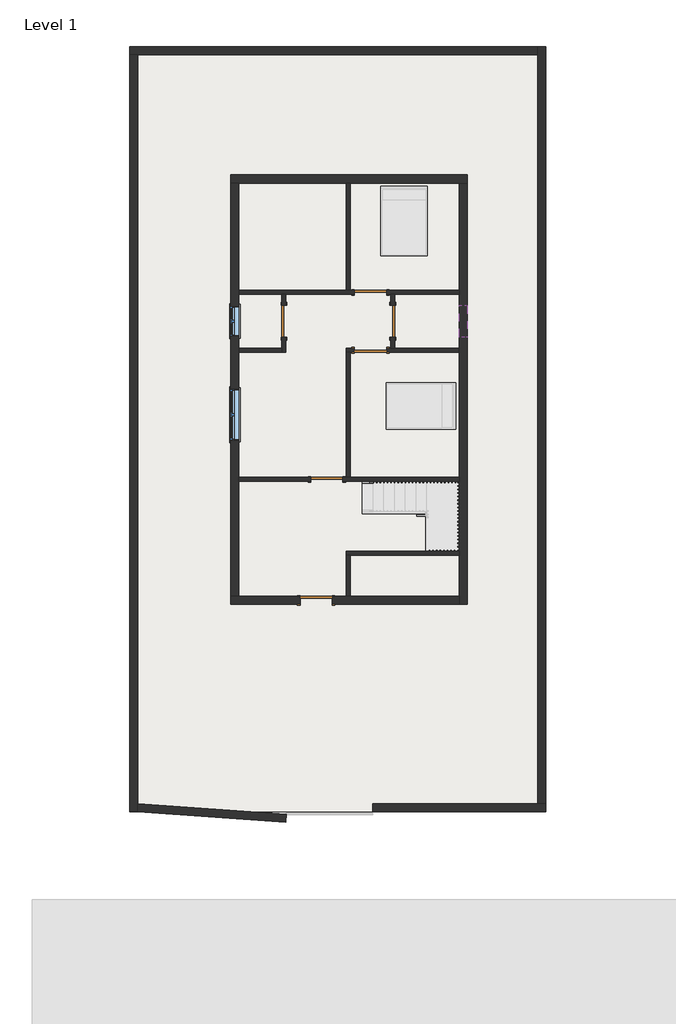
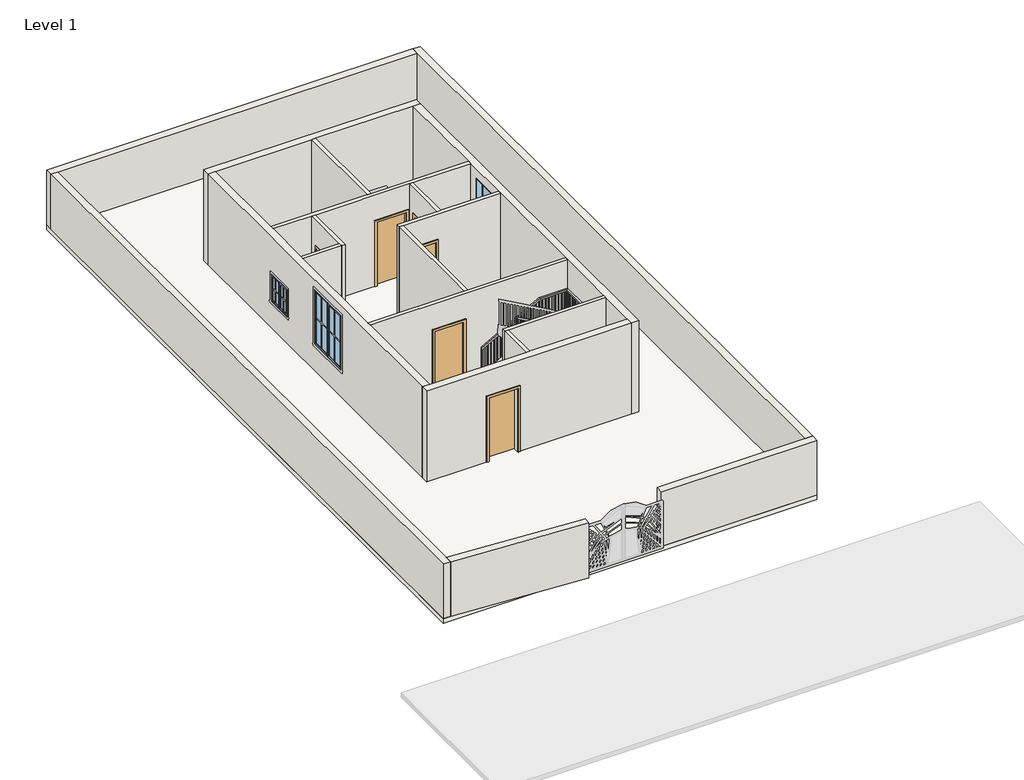
# One storey, part 1 of 2: 19 walls, 6 doors, 3 windows, 1 railing, 1 slab.
"""IFC4 building model written with IfcOpenShell, lengths in millimetres."""

from ifc_helpers import new_model, si_unit, frame, origin, origin_with_axes, place, context, project, spatial, polyline, outline, extrude, faceted_brep, transform, mapped, element, save
from components import door_305aa2a5, door_e5f9f3c4, door_a90ba1ad, window_c1f32544, window_339605e1, window_9ac97e1a

model = new_model("IFC4")

# Units and contexts
model_context = context("Model", 3, world=origin())
ifc_project = project(units=[si_unit("LENGTHUNIT", "METRE", prefix="MILLI")], contexts=[model_context])

# Site, building, storey
site = spatial("IfcSite", under=ifc_project)
building = spatial("IfcBuilding", under=site)
storey = spatial("IfcBuildingStorey", under=building, Name="Level 1", Elevation=0.0)

# Doors
placement = place(None, origin())
door_shape = door_305aa2a5(model_context)
element("IfcDoor", 1, ObjectType="Single-Flush : 36\" x 84\"", at=placement, inside=storey, context=model_context, shape_type="MappedRepresentation", body=[
    mapped(door_shape, transform((-650.940747, 3300.4435985, 0.0), x_axis=(-1.0, 0.0, 0.0), y_axis=(0.0, -1.0, 0.0), z_axis=(0.0, 0.0, 1.0))),
])
element("IfcDoor", 2, ObjectType="Single-Flush : 36\" x 84\"", at=placement, inside=storey, context=model_context, shape_type="MappedRepresentation", body=[
    mapped(door_shape, transform((-22.290747, 2481.2935985, 0.0), x_axis=(0.0, 1.0, 0.0), y_axis=(-1.0, 0.0, 0.0), z_axis=(0.0, 0.0, 1.0))),
])
door_2_shape = door_e5f9f3c4(model_context)
element("IfcDoor", 3, ObjectType="Single-Flush : 36\" x 84\"", at=placement, inside=storey, context=model_context, shape_type="MappedRepresentation", body=[
    mapped(door_2_shape, transform((-650.940747, 1662.1435985, 0.0), x_axis=(-1.0, 0.0, 0.0), y_axis=(0.0, -1.0, 0.0), z_axis=(0.0, 0.0, 1.0))),
])
element("IfcDoor", 4, ObjectType="Single-Flush : 36\" x 84\"", at=placement, inside=storey, context=model_context, shape_type="MappedRepresentation", body=[
    mapped(door_2_shape, transform((-3108.390747, 2481.2935985, 0.0), x_axis=(0.0, 1.0, 0.0), y_axis=(-1.0, 0.0, 0.0), z_axis=(0.0, 0.0, 1.0))),
])
element("IfcDoor", 5, ObjectType="Single-Flush : 36\" x 84\"", at=placement, inside=storey, context=model_context, shape_type="MappedRepresentation", body=[
    mapped(door_2_shape, transform((-1889.190747, -2008.1564015, 0.0), x_axis=(1.0, 0.0, 0.0), y_axis=(0.0, 1.0, 0.0), z_axis=(0.0, 0.0, 1.0))),
])
door_3_shape = door_a90ba1ad(model_context)
element("IfcDoor", 6, ObjectType="Single-Flush : 36\" x 84\"", at=placement, inside=storey, context=model_context, shape_type="MappedRepresentation", body=[
    mapped(door_3_shape, transform((-2193.990747, -5443.5064015, 0.0), x_axis=(-1.0, 0.0, 0.0), y_axis=(0.0, -1.0, 0.0), z_axis=(0.0, 0.0, 1.0))),
])

# Railing
element("IfcRailing", 7, ObjectType="Handrail - Rectangular", at=placement, inside=storey, context=model_context, shape_type="SolidModel", body=[
    faceted_brep([(-879.540747, -2065.3064015, 1083.7333333), (-879.540747, -2065.3064015, 1025.620221), (-879.540747, -2116.1064015, 1025.620221), (-879.540747, -2116.1064015, 1083.7333333), (949.259253, -2065.3064015, 2099.7333333), (962.4228552, -2065.3064015, 2048.9333333), (962.4228552, -2116.1064015, 2048.9333333), (949.259253, -2116.1064015, 2099.7333333), (1863.659253, -2065.3064015, 2099.7333333), (1863.659253, -2065.3064015, 2048.9333333), (1812.859253, -2116.1064015, 2048.9333333), (1812.859253, -2116.1064015, 2099.7333333), (1863.659253, -4046.5064015, 2099.7333333), (1863.659253, -4046.5064015, 2048.9333333), (1812.859253, -3995.7064015, 2048.9333333), (1812.859253, -3995.7064015, 2099.7333333), (1254.059253, -4046.5064015, 2099.7333333), (1240.8956508, -4046.5064015, 2048.9333333), (1240.8956508, -3995.7064015, 2048.9333333), (1254.059253, -3995.7064015, 2099.7333333), (-879.540747, -4046.5064015, 3285.0666667), (-879.540747, -3995.7064015, 3285.0666667), (-879.540747, -3995.7064015, 3226.9535543), (-879.540747, -4046.5064015, 3226.9535543)], [[[0, 1, 2, 3]], [[1, 0, 4, 5]], [[2, 1, 5, 6]], [[3, 2, 6, 7]], [[0, 3, 7, 4]], [[5, 4, 8, 9]], [[6, 5, 9, 10]], [[7, 6, 10, 11]], [[4, 7, 11, 8]], [[9, 8, 12, 13]], [[10, 9, 13, 14]], [[11, 10, 14, 15]], [[8, 11, 15, 12]], [[13, 12, 16, 17]], [[14, 13, 17, 18]], [[15, 14, 18, 19]], [[12, 15, 19, 16]], [[20, 21, 22, 23]], [[17, 16, 20, 23]], [[18, 17, 23, 22]], [[19, 18, 22, 21]], [[16, 19, 21, 20]]]),
    extrude(outline(polyline([(3189.9118876, -812.865747), (2201.3333333, -812.865747), (2201.3333333, -793.815747), (3179.3285543, -793.815747), (3189.9118876, -812.865747)])), frame((0.0, -4030.6314015, 0.0), z_axis=(0.0, 1.0, 0.0), x_axis=(0.0, 0.0, 1.0)), (0.0, 0.0, 1.0), 19.05),
    extrude(outline(polyline([(3133.4674432, -711.265747), (2201.3333333, -711.265747), (2201.3333333, -692.215747), (3122.8841099, -692.215747), (3133.4674432, -711.265747)])), frame((0.0, -4030.6314015, 0.0), z_axis=(0.0, 1.0, 0.0), x_axis=(0.0, 0.0, 1.0)), (0.0, 0.0, 1.0), 19.05),
    extrude(outline(polyline([(3077.0229988, -609.665747), (2201.3333333, -609.665747), (2201.3333333, -590.615747), (3066.4396654, -590.615747), (3077.0229988, -609.665747)])), frame((0.0, -4030.6314015, 0.0), z_axis=(0.0, 1.0, 0.0), x_axis=(0.0, 0.0, 1.0)), (0.0, 0.0, 1.0), 19.05),
    extrude(outline(polyline([(3020.5785543, -508.065747), (2032.0, -508.065747), (2032.0, -489.015747), (3009.995221, -489.015747), (3020.5785543, -508.065747)])), frame((0.0, -4030.6314015, 0.0), z_axis=(0.0, 1.0, 0.0), x_axis=(0.0, 0.0, 1.0)), (0.0, 0.0, 1.0), 19.05),
    extrude(outline(polyline([(2964.1341099, -406.465747), (2032.0, -406.465747), (2032.0, -387.415747), (2953.5507765, -387.415747), (2964.1341099, -406.465747)])), frame((0.0, -4030.6314015, 0.0), z_axis=(0.0, 1.0, 0.0), x_axis=(0.0, 0.0, 1.0)), (0.0, 0.0, 1.0), 19.05),
    extrude(outline(polyline([(2907.6896654, -304.865747), (2032.0, -304.865747), (2032.0, -285.815747), (2897.1063321, -285.815747), (2907.6896654, -304.865747)])), frame((0.0, -4030.6314015, 0.0), z_axis=(0.0, 1.0, 0.0), x_axis=(0.0, 0.0, 1.0)), (0.0, 0.0, 1.0), 19.05),
    extrude(outline(polyline([(2851.245221, -203.265747), (1862.6666667, -203.265747), (1862.6666667, -184.215747), (2840.6618876, -184.215747), (2851.245221, -203.265747)])), frame((0.0, -4030.6314015, 0.0), z_axis=(0.0, 1.0, 0.0), x_axis=(0.0, 0.0, 1.0)), (0.0, 0.0, 1.0), 19.05),
    extrude(outline(polyline([(2794.8007765, -101.665747), (1862.6666667, -101.665747), (1862.6666667, -82.615747), (2784.2174432, -82.615747), (2794.8007765, -101.665747)])), frame((0.0, -4030.6314015, 0.0), z_axis=(0.0, 1.0, 0.0), x_axis=(0.0, 0.0, 1.0)), (0.0, 0.0, 1.0), 19.05),
    extrude(outline(polyline([(2738.3563321, -0.065747), (1862.6666667, -0.065747), (1862.6666667, 18.984253), (2727.7729988, 18.984253), (2738.3563321, -0.065747)])), frame((0.0, -4030.6314015, 0.0), z_axis=(0.0, 1.0, 0.0), x_axis=(0.0, 0.0, 1.0)), (0.0, 0.0, 1.0), 19.05),
    extrude(outline(polyline([(2681.9118876, 101.534253), (1693.3333333, 101.534253), (1693.3333333, 120.584253), (2671.3285543, 120.584253), (2681.9118876, 101.534253)])), frame((0.0, -4030.6314015, 0.0), z_axis=(0.0, 1.0, 0.0), x_axis=(0.0, 0.0, 1.0)), (0.0, 0.0, 1.0), 19.05),
    extrude(outline(polyline([(2625.4674432, 203.134253), (1693.3333333, 203.134253), (1693.3333333, 222.184253), (2614.8841099, 222.184253), (2625.4674432, 203.134253)])), frame((0.0, -4030.6314015, 0.0), z_axis=(0.0, 1.0, 0.0), x_axis=(0.0, 0.0, 1.0)), (0.0, 0.0, 1.0), 19.05),
    extrude(outline(polyline([(2569.0229988, 304.734253), (1693.3333333, 304.734253), (1693.3333333, 323.784253), (2558.4396654, 323.784253), (2569.0229988, 304.734253)])), frame((0.0, -4030.6314015, 0.0), z_axis=(0.0, 1.0, 0.0), x_axis=(0.0, 0.0, 1.0)), (0.0, 0.0, 1.0), 19.05),
    extrude(outline(polyline([(2512.5785543, 406.334253), (1524.0, 406.334253), (1524.0, 425.384253), (2501.995221, 425.384253), (2512.5785543, 406.334253)])), frame((0.0, -4030.6314015, 0.0), z_axis=(0.0, 1.0, 0.0), x_axis=(0.0, 0.0, 1.0)), (0.0, 0.0, 1.0), 19.05),
    extrude(outline(polyline([(2456.1341099, 507.934253), (1524.0, 507.934253), (1524.0, 526.984253), (2445.5507765, 526.984253), (2456.1341099, 507.934253)])), frame((0.0, -4030.6314015, 0.0), z_axis=(0.0, 1.0, 0.0), x_axis=(0.0, 0.0, 1.0)), (0.0, 0.0, 1.0), 19.05),
    extrude(outline(polyline([(2399.6896654, 609.534253), (1524.0, 609.534253), (1524.0, 628.584253), (2389.1063321, 628.584253), (2399.6896654, 609.534253)])), frame((0.0, -4030.6314015, 0.0), z_axis=(0.0, 1.0, 0.0), x_axis=(0.0, 0.0, 1.0)), (0.0, 0.0, 1.0), 19.05),
    extrude(outline(polyline([(2343.245221, 711.134253), (1354.6666667, 711.134253), (1354.6666667, 730.184253), (2332.6618876, 730.184253), (2343.245221, 711.134253)])), frame((0.0, -4030.6314015, 0.0), z_axis=(0.0, 1.0, 0.0), x_axis=(0.0, 0.0, 1.0)), (0.0, 0.0, 1.0), 19.05),
    extrude(outline(polyline([(2286.8007765, 812.734253), (1354.6666667, 812.734253), (1354.6666667, 831.784253), (2276.2174432, 831.784253), (2286.8007765, 812.734253)])), frame((0.0, -4030.6314015, 0.0), z_axis=(0.0, 1.0, 0.0), x_axis=(0.0, 0.0, 1.0)), (0.0, 0.0, 1.0), 19.05),
    extrude(outline(polyline([(2230.3563321, 914.334253), (1354.6666667, 914.334253), (1354.6666667, 933.384253), (2219.7729988, 933.384253), (2230.3563321, 914.334253)])), frame((0.0, -4030.6314015, 0.0), z_axis=(0.0, 1.0, 0.0), x_axis=(0.0, 0.0, 1.0)), (0.0, 0.0, 1.0), 19.05),
    extrude(outline(polyline([(2173.9118876, 1015.934253), (1185.3333333, 1015.934253), (1185.3333333, 1034.984253), (2163.3285543, 1034.984253), (2173.9118876, 1015.934253)])), frame((0.0, -4030.6314015, 0.0), z_axis=(0.0, 1.0, 0.0), x_axis=(0.0, 0.0, 1.0)), (0.0, 0.0, 1.0), 19.05),
    extrude(outline(polyline([(2117.4674432, 1117.534253), (1185.3333333, 1117.534253), (1185.3333333, 1136.584253), (2106.8841099, 1136.584253), (2117.4674432, 1117.534253)])), frame((0.0, -4030.6314015, 0.0), z_axis=(0.0, 1.0, 0.0), x_axis=(0.0, 0.0, 1.0)), (0.0, 0.0, 1.0), 19.05),
    extrude(outline(polyline([(2061.0229988, 1219.134253), (1185.3333333, 1219.134253), (1185.3333333, 1238.184253), (2050.4396654, 1238.184253), (2061.0229988, 1219.134253)])), frame((0.0, -4030.6314015, 0.0), z_axis=(0.0, 1.0, 0.0), x_axis=(0.0, 0.0, 1.0)), (0.0, 0.0, 1.0), 19.05),
    extrude(outline(polyline([(1339.784253, -4030.6314015), (1320.734253, -4030.6314015), (1320.734253, -4011.5814015), (1339.784253, -4011.5814015), (1339.784253, -4030.6314015)])), frame((0.0, 0.0, 1185.3333333), z_axis=(0.0, 0.0, 1.0), x_axis=(1.0, 0.0, 0.0)), (0.0, 0.0, 1.0), 863.6),
    extrude(outline(polyline([(1441.384253, -4030.6314015), (1422.334253, -4030.6314015), (1422.334253, -4011.5814015), (1441.384253, -4011.5814015), (1441.384253, -4030.6314015)])), frame((0.0, 0.0, 1185.3333333), z_axis=(0.0, 0.0, 1.0), x_axis=(1.0, 0.0, 0.0)), (0.0, 0.0, 1.0), 863.6),
    extrude(outline(polyline([(1542.984253, -4030.6314015), (1523.934253, -4030.6314015), (1523.934253, -4011.5814015), (1542.984253, -4011.5814015), (1542.984253, -4030.6314015)])), frame((0.0, 0.0, 1185.3333333), z_axis=(0.0, 0.0, 1.0), x_axis=(1.0, 0.0, 0.0)), (0.0, 0.0, 1.0), 863.6),
    extrude(outline(polyline([(1644.584253, -4030.6314015), (1625.534253, -4030.6314015), (1625.534253, -4011.5814015), (1644.584253, -4011.5814015), (1644.584253, -4030.6314015)])), frame((0.0, 0.0, 1185.3333333), z_axis=(0.0, 0.0, 1.0), x_axis=(1.0, 0.0, 0.0)), (0.0, 0.0, 1.0), 863.6),
    extrude(outline(polyline([(1746.184253, -4030.6314015), (1727.134253, -4030.6314015), (1727.134253, -4011.5814015), (1746.184253, -4011.5814015), (1746.184253, -4030.6314015)])), frame((0.0, 0.0, 1185.3333333), z_axis=(0.0, 0.0, 1.0), x_axis=(1.0, 0.0, 0.0)), (0.0, 0.0, 1.0), 863.6),
    extrude(outline(polyline([(1847.784253, -3909.9814015), (1847.784253, -3929.0314015), (1828.734253, -3929.0314015), (1828.734253, -3909.9814015), (1847.784253, -3909.9814015)])), frame((0.0, 0.0, 1185.3333333), z_axis=(0.0, 0.0, 1.0), x_axis=(1.0, 0.0, 0.0)), (0.0, 0.0, 1.0), 863.6),
    extrude(outline(polyline([(1847.784253, -3808.3814015), (1847.784253, -3827.4314015), (1828.734253, -3827.4314015), (1828.734253, -3808.3814015), (1847.784253, -3808.3814015)])), frame((0.0, 0.0, 1185.3333333), z_axis=(0.0, 0.0, 1.0), x_axis=(1.0, 0.0, 0.0)), (0.0, 0.0, 1.0), 863.6),
    extrude(outline(polyline([(1847.784253, -3706.7814015), (1847.784253, -3725.8314015), (1828.734253, -3725.8314015), (1828.734253, -3706.7814015), (1847.784253, -3706.7814015)])), frame((0.0, 0.0, 1185.3333333), z_axis=(0.0, 0.0, 1.0), x_axis=(1.0, 0.0, 0.0)), (0.0, 0.0, 1.0), 863.6),
    extrude(outline(polyline([(1847.784253, -3605.1814015), (1847.784253, -3624.2314015), (1828.734253, -3624.2314015), (1828.734253, -3605.1814015), (1847.784253, -3605.1814015)])), frame((0.0, 0.0, 1185.3333333), z_axis=(0.0, 0.0, 1.0), x_axis=(1.0, 0.0, 0.0)), (0.0, 0.0, 1.0), 863.6),
    extrude(outline(polyline([(1847.784253, -3503.5814015), (1847.784253, -3522.6314015), (1828.734253, -3522.6314015), (1828.734253, -3503.5814015), (1847.784253, -3503.5814015)])), frame((0.0, 0.0, 1185.3333333), z_axis=(0.0, 0.0, 1.0), x_axis=(1.0, 0.0, 0.0)), (0.0, 0.0, 1.0), 863.6),
    extrude(outline(polyline([(1847.784253, -3401.9814015), (1847.784253, -3421.0314015), (1828.734253, -3421.0314015), (1828.734253, -3401.9814015), (1847.784253, -3401.9814015)])), frame((0.0, 0.0, 1185.3333333), z_axis=(0.0, 0.0, 1.0), x_axis=(1.0, 0.0, 0.0)), (0.0, 0.0, 1.0), 863.6),
    extrude(outline(polyline([(1847.784253, -3300.3814015), (1847.784253, -3319.4314015), (1828.734253, -3319.4314015), (1828.734253, -3300.3814015), (1847.784253, -3300.3814015)])), frame((0.0, 0.0, 1185.3333333), z_axis=(0.0, 0.0, 1.0), x_axis=(1.0, 0.0, 0.0)), (0.0, 0.0, 1.0), 863.6),
    extrude(outline(polyline([(1847.784253, -3198.7814015), (1847.784253, -3217.8314015), (1828.734253, -3217.8314015), (1828.734253, -3198.7814015), (1847.784253, -3198.7814015)])), frame((0.0, 0.0, 1185.3333333), z_axis=(0.0, 0.0, 1.0), x_axis=(1.0, 0.0, 0.0)), (0.0, 0.0, 1.0), 863.6),
    extrude(outline(polyline([(1847.784253, -3097.1814015), (1847.784253, -3116.2314015), (1828.734253, -3116.2314015), (1828.734253, -3097.1814015), (1847.784253, -3097.1814015)])), frame((0.0, 0.0, 1185.3333333), z_axis=(0.0, 0.0, 1.0), x_axis=(1.0, 0.0, 0.0)), (0.0, 0.0, 1.0), 863.6),
    extrude(outline(polyline([(1847.784253, -2995.5814015), (1847.784253, -3014.6314015), (1828.734253, -3014.6314015), (1828.734253, -2995.5814015), (1847.784253, -2995.5814015)])), frame((0.0, 0.0, 1185.3333333), z_axis=(0.0, 0.0, 1.0), x_axis=(1.0, 0.0, 0.0)), (0.0, 0.0, 1.0), 863.6),
    extrude(outline(polyline([(1847.784253, -2893.9814015), (1847.784253, -2913.0314015), (1828.734253, -2913.0314015), (1828.734253, -2893.9814015), (1847.784253, -2893.9814015)])), frame((0.0, 0.0, 1185.3333333), z_axis=(0.0, 0.0, 1.0), x_axis=(1.0, 0.0, 0.0)), (0.0, 0.0, 1.0), 863.6),
    extrude(outline(polyline([(1847.784253, -2792.3814015), (1847.784253, -2811.4314015), (1828.734253, -2811.4314015), (1828.734253, -2792.3814015), (1847.784253, -2792.3814015)])), frame((0.0, 0.0, 1185.3333333), z_axis=(0.0, 0.0, 1.0), x_axis=(1.0, 0.0, 0.0)), (0.0, 0.0, 1.0), 863.6),
    extrude(outline(polyline([(1847.784253, -2690.7814015), (1847.784253, -2709.8314015), (1828.734253, -2709.8314015), (1828.734253, -2690.7814015), (1847.784253, -2690.7814015)])), frame((0.0, 0.0, 1185.3333333), z_axis=(0.0, 0.0, 1.0), x_axis=(1.0, 0.0, 0.0)), (0.0, 0.0, 1.0), 863.6),
    extrude(outline(polyline([(1847.784253, -2589.1814015), (1847.784253, -2608.2314015), (1828.734253, -2608.2314015), (1828.734253, -2589.1814015), (1847.784253, -2589.1814015)])), frame((0.0, 0.0, 1185.3333333), z_axis=(0.0, 0.0, 1.0), x_axis=(1.0, 0.0, 0.0)), (0.0, 0.0, 1.0), 863.6),
    extrude(outline(polyline([(1847.784253, -2487.5814015), (1847.784253, -2506.6314015), (1828.734253, -2506.6314015), (1828.734253, -2487.5814015), (1847.784253, -2487.5814015)])), frame((0.0, 0.0, 1185.3333333), z_axis=(0.0, 0.0, 1.0), x_axis=(1.0, 0.0, 0.0)), (0.0, 0.0, 1.0), 863.6),
    extrude(outline(polyline([(1847.784253, -2385.9814015), (1847.784253, -2405.0314015), (1828.734253, -2405.0314015), (1828.734253, -2385.9814015), (1847.784253, -2385.9814015)])), frame((0.0, 0.0, 1185.3333333), z_axis=(0.0, 0.0, 1.0), x_axis=(1.0, 0.0, 0.0)), (0.0, 0.0, 1.0), 863.6),
    extrude(outline(polyline([(1847.784253, -2284.3814015), (1847.784253, -2303.4314015), (1828.734253, -2303.4314015), (1828.734253, -2284.3814015), (1847.784253, -2284.3814015)])), frame((0.0, 0.0, 1185.3333333), z_axis=(0.0, 0.0, 1.0), x_axis=(1.0, 0.0, 0.0)), (0.0, 0.0, 1.0), 863.6),
    extrude(outline(polyline([(1847.784253, -2182.7814015), (1847.784253, -2201.8314015), (1828.734253, -2201.8314015), (1828.734253, -2182.7814015), (1847.784253, -2182.7814015)])), frame((0.0, 0.0, 1185.3333333), z_axis=(0.0, 0.0, 1.0), x_axis=(1.0, 0.0, 0.0)), (0.0, 0.0, 1.0), 863.6),
    extrude(outline(polyline([(1752.534253, -2081.1814015), (1771.584253, -2081.1814015), (1771.584253, -2100.2314015), (1752.534253, -2100.2314015), (1752.534253, -2081.1814015)])), frame((0.0, 0.0, 1185.3333333), z_axis=(0.0, 0.0, 1.0), x_axis=(1.0, 0.0, 0.0)), (0.0, 0.0, 1.0), 863.6),
    extrude(outline(polyline([(1650.934253, -2081.1814015), (1669.984253, -2081.1814015), (1669.984253, -2100.2314015), (1650.934253, -2100.2314015), (1650.934253, -2081.1814015)])), frame((0.0, 0.0, 1185.3333333), z_axis=(0.0, 0.0, 1.0), x_axis=(1.0, 0.0, 0.0)), (0.0, 0.0, 1.0), 863.6),
    extrude(outline(polyline([(1549.334253, -2081.1814015), (1568.384253, -2081.1814015), (1568.384253, -2100.2314015), (1549.334253, -2100.2314015), (1549.334253, -2081.1814015)])), frame((0.0, 0.0, 1185.3333333), z_axis=(0.0, 0.0, 1.0), x_axis=(1.0, 0.0, 0.0)), (0.0, 0.0, 1.0), 863.6),
    extrude(outline(polyline([(1447.734253, -2081.1814015), (1466.784253, -2081.1814015), (1466.784253, -2100.2314015), (1447.734253, -2100.2314015), (1447.734253, -2081.1814015)])), frame((0.0, 0.0, 1185.3333333), z_axis=(0.0, 0.0, 1.0), x_axis=(1.0, 0.0, 0.0)), (0.0, 0.0, 1.0), 863.6),
    extrude(outline(polyline([(1346.134253, -2081.1814015), (1365.184253, -2081.1814015), (1365.184253, -2100.2314015), (1346.134253, -2100.2314015), (1346.134253, -2081.1814015)])), frame((0.0, 0.0, 1185.3333333), z_axis=(0.0, 0.0, 1.0), x_axis=(1.0, 0.0, 0.0)), (0.0, 0.0, 1.0), 863.6),
    extrude(outline(polyline([(1244.534253, -2081.1814015), (1263.584253, -2081.1814015), (1263.584253, -2100.2314015), (1244.534253, -2100.2314015), (1244.534253, -2081.1814015)])), frame((0.0, 0.0, 1185.3333333), z_axis=(0.0, 0.0, 1.0), x_axis=(1.0, 0.0, 0.0)), (0.0, 0.0, 1.0), 863.6),
    extrude(outline(polyline([(1142.934253, -2081.1814015), (1161.984253, -2081.1814015), (1161.984253, -2100.2314015), (1142.934253, -2100.2314015), (1142.934253, -2081.1814015)])), frame((0.0, 0.0, 1185.3333333), z_axis=(0.0, 0.0, 1.0), x_axis=(1.0, 0.0, 0.0)), (0.0, 0.0, 1.0), 863.6),
    extrude(outline(polyline([(1041.334253, -2081.1814015), (1060.384253, -2081.1814015), (1060.384253, -2100.2314015), (1041.334253, -2100.2314015), (1041.334253, -2081.1814015)])), frame((0.0, 0.0, 1185.3333333), z_axis=(0.0, 0.0, 1.0), x_axis=(1.0, 0.0, 0.0)), (0.0, 0.0, 1.0), 863.6),
    extrude(outline(polyline([(2036.3285543, 939.734253), (1185.3333333, 939.734253), (1185.3333333, 958.784253), (2046.9118876, 958.784253), (2036.3285543, 939.734253)])), frame((0.0, -2100.2314015, 0.0), z_axis=(0.0, 1.0, 0.0), x_axis=(0.0, 0.0, 1.0)), (0.0, 0.0, 1.0), 19.05),
    extrude(outline(polyline([(1979.8841099, 838.134253), (1016.0, 838.134253), (1016.0, 857.184253), (1990.4674432, 857.184253), (1979.8841099, 838.134253)])), frame((0.0, -2100.2314015, 0.0), z_axis=(0.0, 1.0, 0.0), x_axis=(0.0, 0.0, 1.0)), (0.0, 0.0, 1.0), 19.05),
    extrude(outline(polyline([(1923.4396654, 736.534253), (1016.0, 736.534253), (1016.0, 755.584253), (1934.0229988, 755.584253), (1923.4396654, 736.534253)])), frame((0.0, -2100.2314015, 0.0), z_axis=(0.0, 1.0, 0.0), x_axis=(0.0, 0.0, 1.0)), (0.0, 0.0, 1.0), 19.05),
    extrude(outline(polyline([(1866.995221, 634.934253), (1016.0, 634.934253), (1016.0, 653.984253), (1877.5785543, 653.984253), (1866.995221, 634.934253)])), frame((0.0, -2100.2314015, 0.0), z_axis=(0.0, 1.0, 0.0), x_axis=(0.0, 0.0, 1.0)), (0.0, 0.0, 1.0), 19.05),
    extrude(outline(polyline([(1810.5507765, 533.334253), (846.6666667, 533.334253), (846.6666667, 552.384253), (1821.1341099, 552.384253), (1810.5507765, 533.334253)])), frame((0.0, -2100.2314015, 0.0), z_axis=(0.0, 1.0, 0.0), x_axis=(0.0, 0.0, 1.0)), (0.0, 0.0, 1.0), 19.05),
    extrude(outline(polyline([(1754.1063321, 431.734253), (846.6666667, 431.734253), (846.6666667, 450.784253), (1764.6896654, 450.784253), (1754.1063321, 431.734253)])), frame((0.0, -2100.2314015, 0.0), z_axis=(0.0, 1.0, 0.0), x_axis=(0.0, 0.0, 1.0)), (0.0, 0.0, 1.0), 19.05),
    extrude(outline(polyline([(1697.6618876, 330.134253), (846.6666667, 330.134253), (846.6666667, 349.184253), (1708.245221, 349.184253), (1697.6618876, 330.134253)])), frame((0.0, -2100.2314015, 0.0), z_axis=(0.0, 1.0, 0.0), x_axis=(0.0, 0.0, 1.0)), (0.0, 0.0, 1.0), 19.05),
    extrude(outline(polyline([(1641.2174432, 228.534253), (677.3333333, 228.534253), (677.3333333, 247.584253), (1651.8007765, 247.584253), (1641.2174432, 228.534253)])), frame((0.0, -2100.2314015, 0.0), z_axis=(0.0, 1.0, 0.0), x_axis=(0.0, 0.0, 1.0)), (0.0, 0.0, 1.0), 19.05),
    extrude(outline(polyline([(1584.7729988, 126.934253), (677.3333333, 126.934253), (677.3333333, 145.984253), (1595.3563321, 145.984253), (1584.7729988, 126.934253)])), frame((0.0, -2100.2314015, 0.0), z_axis=(0.0, 1.0, 0.0), x_axis=(0.0, 0.0, 1.0)), (0.0, 0.0, 1.0), 19.05),
    extrude(outline(polyline([(1528.3285543, 25.334253), (677.3333333, 25.334253), (677.3333333, 44.384253), (1538.9118876, 44.384253), (1528.3285543, 25.334253)])), frame((0.0, -2100.2314015, 0.0), z_axis=(0.0, 1.0, 0.0), x_axis=(0.0, 0.0, 1.0)), (0.0, 0.0, 1.0), 19.05),
    extrude(outline(polyline([(1471.8841099, -76.265747), (508.0, -76.265747), (508.0, -57.215747), (1482.4674432, -57.215747), (1471.8841099, -76.265747)])), frame((0.0, -2100.2314015, 0.0), z_axis=(0.0, 1.0, 0.0), x_axis=(0.0, 0.0, 1.0)), (0.0, 0.0, 1.0), 19.05),
    extrude(outline(polyline([(1415.4396654, -177.865747), (508.0, -177.865747), (508.0, -158.815747), (1426.0229988, -158.815747), (1415.4396654, -177.865747)])), frame((0.0, -2100.2314015, 0.0), z_axis=(0.0, 1.0, 0.0), x_axis=(0.0, 0.0, 1.0)), (0.0, 0.0, 1.0), 19.05),
    extrude(outline(polyline([(1358.995221, -279.465747), (508.0, -279.465747), (508.0, -260.415747), (1369.5785543, -260.415747), (1358.995221, -279.465747)])), frame((0.0, -2100.2314015, 0.0), z_axis=(0.0, 1.0, 0.0), x_axis=(0.0, 0.0, 1.0)), (0.0, 0.0, 1.0), 19.05),
    extrude(outline(polyline([(1302.5507765, -381.065747), (338.6666667, -381.065747), (338.6666667, -362.015747), (1313.1341099, -362.015747), (1302.5507765, -381.065747)])), frame((0.0, -2100.2314015, 0.0), z_axis=(0.0, 1.0, 0.0), x_axis=(0.0, 0.0, 1.0)), (0.0, 0.0, 1.0), 19.05),
    extrude(outline(polyline([(1246.1063321, -482.665747), (338.6666667, -482.665747), (338.6666667, -463.615747), (1256.6896654, -463.615747), (1246.1063321, -482.665747)])), frame((0.0, -2100.2314015, 0.0), z_axis=(0.0, 1.0, 0.0), x_axis=(0.0, 0.0, 1.0)), (0.0, 0.0, 1.0), 19.05),
    extrude(outline(polyline([(1189.6618876, -584.265747), (338.6666667, -584.265747), (338.6666667, -565.215747), (1200.245221, -565.215747), (1189.6618876, -584.265747)])), frame((0.0, -2100.2314015, 0.0), z_axis=(0.0, 1.0, 0.0), x_axis=(0.0, 0.0, 1.0)), (0.0, 0.0, 1.0), 19.05),
    extrude(outline(polyline([(1133.2174432, -685.865747), (169.3333333, -685.865747), (169.3333333, -666.815747), (1143.8007765, -666.815747), (1133.2174432, -685.865747)])), frame((0.0, -2100.2314015, 0.0), z_axis=(0.0, 1.0, 0.0), x_axis=(0.0, 0.0, 1.0)), (0.0, 0.0, 1.0), 19.05),
    extrude(outline(polyline([(1076.7729988, -787.465747), (169.3333333, -787.465747), (169.3333333, -768.415747), (1087.3563321, -768.415747), (1076.7729988, -787.465747)])), frame((0.0, -2100.2314015, 0.0), z_axis=(0.0, 1.0, 0.0), x_axis=(0.0, 0.0, 1.0)), (0.0, 0.0, 1.0), 19.05),
    extrude(outline(polyline([(1847.784253, -4011.5814015), (1847.784253, -4030.6314015), (1828.734253, -4030.6314015), (1828.734253, -4011.5814015), (1847.784253, -4011.5814015)])), frame((0.0, 0.0, 1185.3333333), z_axis=(0.0, 0.0, 1.0), x_axis=(1.0, 0.0, 0.0)), (0.0, 0.0, 1.0), 863.6),
    extrude(outline(polyline([(1828.734253, -2081.1814015), (1847.784253, -2081.1814015), (1847.784253, -2100.2314015), (1828.734253, -2100.2314015), (1828.734253, -2081.1814015)])), frame((0.0, 0.0, 1185.3333333), z_axis=(0.0, 0.0, 1.0), x_axis=(1.0, 0.0, 0.0)), (0.0, 0.0, 1.0), 863.6),
    extrude(outline(polyline([(3226.9535543, -879.540747), (2201.3333333, -879.540747), (2201.3333333, -860.490747), (3216.370221, -860.490747), (3226.9535543, -879.540747)])), frame((0.0, -4030.6314015, 0.0), z_axis=(0.0, 1.0, 0.0), x_axis=(0.0, 0.0, 1.0)), (0.0, 0.0, 1.0), 19.05),
    extrude(outline(polyline([(1025.620221, -879.540747), (169.3333333, -879.540747), (169.3333333, -860.490747), (1036.2035543, -860.490747), (1025.620221, -879.540747)])), frame((0.0, -2100.2314015, 0.0), z_axis=(0.0, 1.0, 0.0), x_axis=(0.0, 0.0, 1.0)), (0.0, 0.0, 1.0), 19.05),
])

# Slab
element("IfcSlab", 8, ObjectType="Generic - 12\"", at=placement, inside=storey, context=model_context, shape_type="SweptSolid", body=[
    extrude(outline(polyline([(4327.3334921, 10279.3075002), (4327.3334921, -11437.6924998), (-7483.6665079, -11437.6924998), (-7483.6665079, 10279.3075002), (4327.3334921, 10279.3075002)])), frame((0.0, 0.0, -152.4), z_axis=(0.0, 0.0, 1.0), x_axis=(1.0, 0.0, 0.0)), (0.0, 0.0, 1.0), 152.4),
])

# Walls
element("IfcWall", 9, ObjectType="WALL4.5\"", at=placement, inside=storey, context=model_context, shape_type="SweptSolid", body=[
    extrude(outline(polyline([(-1336.740747, 3357.5935985), (-1336.740747, 6405.5935985), (-1222.440747, 6405.5935985), (-1222.440747, 3357.5935985), (-1336.740747, 3357.5935985)])), origin_with_axes(), (0.0, 0.0, 1.0), 3048.0),
])
element("IfcWall", 10, ObjectType="WALL4.5\"", at=placement, inside=storey, context=model_context, shape_type="Brep", body=[
    faceted_brep([(-4384.740747, 3243.2935985, 0.0), (-3165.540747, 3243.2935985, 0.0), (-3051.240747, 3243.2935985, 0.0), (-1108.140747, 3243.2935985, 0.0), (-1108.140747, 3243.2935985, 2133.6), (-193.740747, 3243.2935985, 2133.6), (-193.740747, 3243.2935985, 0.0), (-79.440747, 3243.2935985, 0.0), (34.859253, 3243.2935985, 0.0), (1863.659253, 3243.2935985, 0.0), (1863.659253, 3243.2935985, 3048.0), (34.859253, 3243.2935985, 3048.0), (-79.440747, 3243.2935985, 3048.0), (-3051.240747, 3243.2935985, 3048.0), (-3165.540747, 3243.2935985, 3048.0), (-4384.740747, 3243.2935985, 3048.0), (-1108.140747, 3357.5935985, 2133.6), (-1108.140747, 3357.5935985, 0.0), (-1222.440747, 3357.5935985, 0.0), (-1336.740747, 3357.5935985, 0.0), (-4384.740747, 3357.5935985, 0.0), (-4384.740747, 3357.5935985, 3048.0), (-1336.740747, 3357.5935985, 3048.0), (-1222.440747, 3357.5935985, 3048.0), (1863.659253, 3357.5935985, 3048.0), (1863.659253, 3357.5935985, 0.0), (-193.740747, 3357.5935985, 0.0), (-193.740747, 3357.5935985, 2133.6)], [[[0, 1, 2, 3, 4, 5, 6, 7, 8, 9, 10, 11, 12, 13, 14, 15]], [[16, 17, 18, 19, 20, 21, 22, 23, 24, 25, 26, 27]], [[26, 25, 9, 8, 7, 6]], [[20, 19, 18, 17, 3, 2, 1, 0]], [[10, 9, 25, 24]], [[0, 15, 21, 20]], [[4, 3, 17, 16]], [[5, 4, 16, 27]], [[6, 5, 27, 26]], [[15, 14, 13, 12, 11, 10, 24, 23, 22, 21]]]),
])
element("IfcWall", 11, ObjectType="WALL4.5\"", at=placement, inside=storey, context=model_context, shape_type="SweptSolid", body=[
    extrude(outline(polyline([(3243.2935985, 0.0), (2938.4935985, 0.0), (2938.4935985, 2133.6), (2024.0935985, 2133.6), (2024.0935985, 0.0), (1719.2935985, 0.0), (1719.2935985, 3048.0), (3243.2935985, 3048.0), (3243.2935985, 0.0)])), frame((-79.440747, 0.0, 0.0), z_axis=(1.0, 0.0, 0.0), x_axis=(0.0, 1.0, 0.0)), (0.0, 0.0, 1.0), 114.3),
])
element("IfcWall", 12, ObjectType="WALL4.5\"", at=placement, inside=storey, context=model_context, shape_type="Brep", body=[
    faceted_brep([(-1108.140747, 1719.2935985, 2133.6), (-1108.140747, 1719.2935985, 0.0), (-1336.740747, 1719.2935985, 0.0), (-1336.740747, 1719.2935985, 3048.0), (-79.440747, 1719.2935985, 3048.0), (34.859253, 1719.2935985, 3048.0), (1863.659253, 1719.2935985, 3048.0), (1863.659253, 1719.2935985, 0.0), (34.859253, 1719.2935985, 0.0), (-79.440747, 1719.2935985, 0.0), (-193.740747, 1719.2935985, 0.0), (-193.740747, 1719.2935985, 2133.6), (-1336.740747, 1604.9935985, 0.0), (-1222.440747, 1604.9935985, 0.0), (-1108.140747, 1604.9935985, 0.0), (-1108.140747, 1604.9935985, 2133.6), (-193.740747, 1604.9935985, 2133.6), (-193.740747, 1604.9935985, 0.0), (1863.659253, 1604.9935985, 0.0), (1863.659253, 1604.9935985, 3048.0), (-1222.440747, 1604.9935985, 3048.0), (-1336.740747, 1604.9935985, 3048.0)], [[[0, 1, 2, 3, 4, 5, 6, 7, 8, 9, 10, 11]], [[12, 13, 14, 15, 16, 17, 18, 19, 20, 21]], [[2, 1, 14, 13, 12]], [[10, 9, 8, 7, 18, 17]], [[7, 6, 19, 18]], [[3, 2, 12, 21]], [[15, 14, 1, 0]], [[16, 15, 0, 11]], [[17, 16, 11, 10]], [[6, 5, 4, 3, 21, 20, 19]]]),
])
element("IfcWall", 13, ObjectType="WALL4.5\"", at=placement, inside=storey, context=model_context, shape_type="SweptSolid", body=[
    extrude(outline(polyline([(-1336.740747, -1951.0064015), (-1336.740747, 1604.9935985), (-1222.440747, 1604.9935985), (-1222.440747, -1951.0064015), (-1336.740747, -1951.0064015)])), origin_with_axes(), (0.0, 0.0, 1.0), 3048.0),
])
element("IfcWall", 14, ObjectType="WALL4.5\"", at=placement, inside=storey, context=model_context, shape_type="Brep", body=[
    faceted_brep([(-3165.540747, 3243.2935985, 0.0), (-3165.540747, 2938.4935985, 0.0), (-3165.540747, 2938.4935985, 2133.6), (-3165.540747, 2024.0935985, 2133.6), (-3165.540747, 2024.0935985, 0.0), (-3165.540747, 1719.2935985, 0.0), (-3165.540747, 1604.9935985, 0.0), (-3165.540747, 1604.9935985, 3048.0), (-3165.540747, 1719.2935985, 3048.0), (-3165.540747, 3243.2935985, 3048.0), (-3051.240747, 2938.4935985, 2133.6), (-3051.240747, 2938.4935985, 0.0), (-3051.240747, 3243.2935985, 0.0), (-3051.240747, 3243.2935985, 3048.0), (-3051.240747, 1604.9935985, 3048.0), (-3051.240747, 1604.9935985, 0.0), (-3051.240747, 2024.0935985, 0.0), (-3051.240747, 2024.0935985, 2133.6)], [[[0, 1, 2, 3, 4, 5, 6, 7, 8, 9]], [[10, 11, 12, 13, 14, 15, 16, 17]], [[16, 15, 6, 5, 4]], [[12, 11, 1, 0]], [[0, 9, 13, 12]], [[7, 6, 15, 14]], [[2, 1, 11, 10]], [[3, 2, 10, 17]], [[4, 3, 17, 16]], [[9, 8, 7, 14, 13]]]),
])
element("IfcWall", 15, ObjectType="WALL4.5\"", at=placement, inside=storey, context=model_context, shape_type="SweptSolid", body=[
    extrude(outline(polyline([(-4384.740747, 1719.2935985), (-3165.540747, 1719.2935985), (-3165.540747, 1604.9935985), (-4384.740747, 1604.9935985), (-4384.740747, 1719.2935985)])), origin_with_axes(), (0.0, 0.0, 1.0), 3048.0),
])
element("IfcWall", 16, ObjectType="WALL4.5\"", at=placement, inside=storey, context=model_context, shape_type="Brep", body=[
    faceted_brep([(-1431.990747, -2065.3064015, 2133.6), (-1431.990747, -2065.3064015, 0.0), (1863.659253, -2065.3064015, 0.0), (1863.659253, -2065.3064015, 3048.0), (-4384.740747, -2065.3064015, 3048.0), (-4384.740747, -2065.3064015, 0.0), (-2346.390747, -2065.3064015, 0.0), (-2346.390747, -2065.3064015, 2133.6), (1863.659253, -1951.0064015, 0.0), (-1222.440747, -1951.0064015, 0.0), (-1336.740747, -1951.0064015, 0.0), (-1431.990747, -1951.0064015, 0.0), (-1431.990747, -1951.0064015, 2133.6), (-2346.390747, -1951.0064015, 2133.6), (-2346.390747, -1951.0064015, 0.0), (-4384.740747, -1951.0064015, 0.0), (-4384.740747, -1951.0064015, 3048.0), (-1336.740747, -1951.0064015, 3048.0), (-1222.440747, -1951.0064015, 3048.0), (1863.659253, -1951.0064015, 3048.0)], [[[0, 1, 2, 3, 4, 5, 6, 7]], [[8, 9, 10, 11, 12, 13, 14, 15, 16, 17, 18, 19]], [[6, 5, 15, 14]], [[2, 1, 11, 10, 9, 8]], [[3, 2, 8, 19]], [[5, 4, 16, 15]], [[12, 11, 1, 0]], [[13, 12, 0, 7]], [[14, 13, 7, 6]], [[4, 3, 19, 18, 17, 16]]]),
])
element("IfcWall", 17, ObjectType="WALL4.5\"", at=placement, inside=storey, context=model_context, shape_type="Brep", body=[
    faceted_brep([(1863.659253, -4046.5064015, 0.0), (-1336.740747, -4046.5064015, 0.0), (-1336.740747, -4046.5064015, 3048.0), (1863.659253, -4046.5064015, 3048.0), (1863.659253, -4160.8064015, 0.0), (1863.659253, -4160.8064015, 3048.0), (-1222.440747, -4160.8064015, 3048.0), (-1336.740747, -4160.8064015, 3048.0), (-1336.740747, -4160.8064015, 0.0), (-1222.440747, -4160.8064015, 0.0)], [[[0, 1, 2, 3]], [[4, 5, 6, 7, 8, 9]], [[1, 0, 4, 9, 8]], [[0, 3, 5, 4]], [[2, 1, 8, 7]], [[3, 2, 7, 6, 5]]]),
])
element("IfcWall", 18, ObjectType="WALL4.5\"", at=placement, inside=storey, context=model_context, shape_type="SweptSolid", body=[
    extrude(outline(polyline([(-1336.740747, -5329.2064015), (-1336.740747, -4160.8064015), (-1222.440747, -4160.8064015), (-1222.440747, -5329.2064015), (-1336.740747, -5329.2064015)])), origin_with_axes(), (0.0, 0.0, 1.0), 3048.0),
])
element("IfcWall", 19, ObjectType="WALL9\"", at=placement, inside=storey, context=model_context, shape_type="Brep", body=[
    faceted_brep([(-4613.340747, 6405.5935985, 0.0), (-4384.740747, 6405.5935985, 0.0), (-1336.740747, 6405.5935985, 0.0), (-1222.440747, 6405.5935985, 0.0), (1863.659253, 6405.5935985, 0.0), (2092.259253, 6405.5935985, 0.0), (2092.259253, 6405.5935985, 3048.0), (1863.659253, 6405.5935985, 3048.0), (-1222.440747, 6405.5935985, 3048.0), (-1336.740747, 6405.5935985, 3048.0), (-4384.740747, 6405.5935985, 3048.0), (-4613.340747, 6405.5935985, 3048.0), (-4613.340747, 6634.1935985, 0.0), (-4613.340747, 6634.1935985, 3048.0), (2092.259253, 6634.1935985, 3048.0), (2092.259253, 6634.1935985, 0.0)], [[[0, 1, 2, 3, 4, 5, 6, 7, 8, 9, 10, 11]], [[12, 13, 14, 15]], [[5, 4, 3, 2, 1, 0, 12, 15]], [[6, 5, 15, 14]], [[0, 11, 13, 12]], [[11, 10, 9, 8, 7, 6, 14, 13]]]),
])
element("IfcWall", 20, ObjectType="WALL9\"", at=placement, inside=storey, context=model_context, shape_type="Brep", body=[
    faceted_brep([(1863.659253, 6405.5935985, 0.0), (1863.659253, 3357.5935985, 0.0), (1863.659253, 3243.2935985, 0.0), (1863.659253, 1719.2935985, 0.0), (1863.659253, 1604.9935985, 0.0), (1863.659253, -1951.0064015, 0.0), (1863.659253, -2065.3064015, 0.0), (1863.659253, -4046.5064015, 0.0), (1863.659253, -4160.8064015, 0.0), (1863.659253, -5329.2064015, 0.0), (1863.659253, -5557.8064015, 0.0), (1863.659253, -5557.8064015, 3048.0), (1863.659253, -5329.2064015, 3048.0), (1863.659253, -4160.8064015, 3048.0), (1863.659253, -4046.5064015, 3048.0), (1863.659253, -2065.3064015, 3048.0), (1863.659253, -1951.0064015, 3048.0), (1863.659253, 1604.9935985, 3048.0), (1863.659253, 1719.2935985, 3048.0), (1863.659253, 3243.2935985, 3048.0), (1863.659253, 3357.5935985, 3048.0), (1863.659253, 6405.5935985, 3048.0), (1863.659253, 2024.0935985, 2743.2), (1863.659253, 2024.0935985, 1524.0), (1863.659253, 2938.4935985, 1524.0), (1863.659253, 2938.4935985, 2743.2), (2092.259253, 6405.5935985, 0.0), (2092.259253, 6405.5935985, 3048.0), (2092.259253, -5557.8064015, 3048.0), (2092.259253, -5557.8064015, 0.0), (2092.259253, 2024.0935985, 2743.2), (2092.259253, 2938.4935985, 2743.2), (2092.259253, 2938.4935985, 1524.0), (2092.259253, 2024.0935985, 1524.0)], [[[0, 1, 2, 3, 4, 5, 6, 7, 8, 9, 10, 11, 12, 13, 14, 15, 16, 17, 18, 19, 20, 21], [22, 23, 24, 25]], [[26, 27, 28, 29], [30, 31, 32, 33]], [[10, 9, 8, 7, 6, 5, 4, 3, 2, 1, 0, 26, 29]], [[0, 21, 27, 26]], [[11, 10, 29, 28]], [[23, 22, 30, 33]], [[24, 23, 33, 32]], [[25, 24, 32, 31]], [[22, 25, 31, 30]], [[21, 20, 19, 18, 17, 16, 15, 14, 13, 12, 11, 28, 27]]]),
])
element("IfcWall", 21, ObjectType="WALL9\"", at=placement, inside=storey, context=model_context, shape_type="Brep", body=[
    faceted_brep([(-2651.190747, -5329.2064015, 2133.6), (-2651.190747, -5329.2064015, 0.0), (-4384.740747, -5329.2064015, 0.0), (-4613.340747, -5329.2064015, 0.0), (-4613.340747, -5329.2064015, 3048.0), (-4384.740747, -5329.2064015, 3048.0), (-1336.740747, -5329.2064015, 3048.0), (-1222.440747, -5329.2064015, 3048.0), (1863.659253, -5329.2064015, 3048.0), (1863.659253, -5329.2064015, 0.0), (-1222.440747, -5329.2064015, 0.0), (-1336.740747, -5329.2064015, 0.0), (-1736.790747, -5329.2064015, 0.0), (-1736.790747, -5329.2064015, 2133.6), (-4613.340747, -5557.8064015, 0.0), (-2651.190747, -5557.8064015, 0.0), (-2651.190747, -5557.8064015, 2133.6), (-1736.790747, -5557.8064015, 2133.6), (-1736.790747, -5557.8064015, 0.0), (1863.659253, -5557.8064015, 0.0), (1863.659253, -5557.8064015, 3048.0), (-4613.340747, -5557.8064015, 3048.0)], [[[0, 1, 2, 3, 4, 5, 6, 7, 8, 9, 10, 11, 12, 13]], [[14, 15, 16, 17, 18, 19, 20, 21]], [[3, 2, 1, 15, 14]], [[12, 11, 10, 9, 19, 18]], [[9, 8, 20, 19]], [[4, 3, 14, 21]], [[16, 15, 1, 0]], [[17, 16, 0, 13]], [[18, 17, 13, 12]], [[8, 7, 6, 5, 4, 21, 20]]]),
])
element("IfcWall", 22, ObjectType="WALL9\"", at=placement, inside=storey, context=model_context, shape_type="Brep", body=[
    faceted_brep([(-4384.740747, -5329.2064015, 0.0), (-4384.740747, -2065.3064015, 0.0), (-4384.740747, -1951.0064015, 0.0), (-4384.740747, 1604.9935985, 0.0), (-4384.740747, 1719.2935985, 0.0), (-4384.740747, 3243.2935985, 0.0), (-4384.740747, 3357.5935985, 0.0), (-4384.740747, 6405.5935985, 0.0), (-4384.740747, 6405.5935985, 3048.0), (-4384.740747, 3357.5935985, 3048.0), (-4384.740747, 3243.2935985, 3048.0), (-4384.740747, 1719.2935985, 3048.0), (-4384.740747, 1604.9935985, 3048.0), (-4384.740747, -1951.0064015, 3048.0), (-4384.740747, -2065.3064015, 3048.0), (-4384.740747, -5329.2064015, 3048.0), (-4384.740747, 550.8935985, 2743.2), (-4384.740747, 550.8935985, 914.4), (-4384.740747, -896.9064015, 914.4), (-4384.740747, -896.9064015, 2743.2), (-4384.740747, 2913.0935985, 1828.8), (-4384.740747, 2913.0935985, 914.4), (-4384.740747, 2049.4935985, 914.4), (-4384.740747, 2049.4935985, 1828.8), (-4613.340747, -5329.2064015, 0.0), (-4613.340747, -5329.2064015, 3048.0), (-4613.340747, 6405.5935985, 3048.0), (-4613.340747, 6405.5935985, 0.0), (-4613.340747, 550.8935985, 2743.2), (-4613.340747, -896.9064015, 2743.2), (-4613.340747, -896.9064015, 914.4), (-4613.340747, 550.8935985, 914.4), (-4613.340747, 2913.0935985, 1828.8), (-4613.340747, 2049.4935985, 1828.8), (-4613.340747, 2049.4935985, 914.4), (-4613.340747, 2913.0935985, 914.4)], [[[0, 1, 2, 3, 4, 5, 6, 7, 8, 9, 10, 11, 12, 13, 14, 15], [16, 17, 18, 19], [20, 21, 22, 23]], [[24, 25, 26, 27], [28, 29, 30, 31], [32, 33, 34, 35]], [[7, 6, 5, 4, 3, 2, 1, 0, 24, 27]], [[8, 7, 27, 26]], [[0, 15, 25, 24]], [[17, 16, 28, 31]], [[18, 17, 31, 30]], [[19, 18, 30, 29]], [[16, 19, 29, 28]], [[21, 20, 32, 35]], [[22, 21, 35, 34]], [[23, 22, 34, 33]], [[20, 23, 33, 32]], [[15, 14, 13, 12, 11, 10, 9, 8, 26, 25]]]),
])
element("IfcWall", 23, ObjectType="WALL9\"", at=placement, inside=storey, context=model_context, shape_type="Brep", body=[
    faceted_brep([(-7483.6665079, 10050.7075002, 0.0), (-7255.0665079, 10050.7075002, 0.0), (4098.7334921, 10050.7075002, 0.0), (4098.7334921, 10050.7075002, 1828.8), (-7255.0665079, 10050.7075002, 1828.8), (-7483.6665079, 10050.7075002, 1828.8), (-7483.6665079, 10279.3075002, 0.0), (-7483.6665079, 10279.3075002, 1828.8), (4098.7334921, 10279.3075002, 1828.8), (4098.7334921, 10279.3075002, 0.0)], [[[0, 1, 2, 3, 4, 5]], [[6, 7, 8, 9]], [[2, 1, 0, 6, 9]], [[5, 4, 3, 8, 7]], [[0, 5, 7, 6]], [[3, 2, 9, 8]]]),
])
element("IfcWall", 24, ObjectType="WALL9\"", at=placement, inside=storey, context=model_context, shape_type="Brep", body=[
    faceted_brep([(-7255.0665079, -11446.2433523, 0.0), (-7255.0665079, -11217.0851344, 0.0), (-7255.0665079, 10050.7075002, 0.0), (-7255.0665079, 10050.7075002, 1828.8), (-7255.0665079, -11217.0851344, 1828.8), (-7255.0665079, -11446.2433523, 1828.8), (-7483.6665079, -11430.2580831, 0.0), (-7483.6665079, -11430.2580831, 1828.8), (-7483.6665079, 10050.7075002, 1828.8), (-7483.6665079, 10050.7075002, 0.0)], [[[0, 1, 2, 3, 4, 5]], [[6, 7, 8, 9]], [[2, 1, 0, 6, 9]], [[5, 4, 3, 8, 7]], [[0, 5, 7, 6]], [[3, 2, 9, 8]]]),
])
element("IfcWall", 25, ObjectType="WALL9\"", at=placement, inside=storey, context=model_context, shape_type="Brep", body=[
    faceted_brep([(4327.3334921, -11209.0924998, 0.0), (4098.7334921, -11209.0924998, 0.0), (-587.5665079, -11209.0924998, 0.0), (-587.5665079, -11209.0924998, 1828.8), (4098.7334921, -11209.0924998, 1828.8), (4327.3334921, -11209.0924998, 1828.8), (4327.3334921, -11437.6924998, 0.0), (4327.3334921, -11437.6924998, 1828.8), (-587.5665079, -11437.6924998, 1828.8), (-587.5665079, -11437.6924998, 0.0)], [[[0, 1, 2, 3, 4, 5]], [[6, 7, 8, 9]], [[2, 1, 0, 6, 9]], [[3, 2, 9, 8]], [[5, 4, 3, 8, 7]], [[0, 5, 7, 6]]]),
])
element("IfcWall", 26, ObjectType="WALL9\"", at=placement, inside=storey, context=model_context, shape_type="Brep", body=[
    faceted_brep([(4098.7334921, 10279.3075002, 0.0), (4098.7334921, 10050.7075002, 0.0), (4098.7334921, -11209.0924998, 0.0), (4098.7334921, -11209.0924998, 1828.8), (4098.7334921, 10050.7075002, 1828.8), (4098.7334921, 10279.3075002, 1828.8), (4327.3334921, 10279.3075002, 0.0), (4327.3334921, 10279.3075002, 1828.8), (4327.3334921, -11209.0924998, 1828.8), (4327.3334921, -11209.0924998, 0.0)], [[[0, 1, 2, 3, 4, 5]], [[6, 7, 8, 9]], [[2, 1, 0, 6, 9]], [[5, 4, 3, 8, 7]], [[0, 5, 7, 6]], [[3, 2, 9, 8]]]),
])
element("IfcWall", 27, ObjectType="WALL9\"", at=placement, inside=storey, context=model_context, shape_type="SweptSolid", body=[
    extrude(outline(polyline([(-7255.0665079, -11217.0851344), (-3036.546812, -11512.0727679), (-3052.4931419, -11740.1159098), (-7255.0665079, -11446.2433523), (-7255.0665079, -11217.0851344)])), origin_with_axes(), (0.0, 0.0, 1.0), 1828.8),
])

# Windows
window_shape = window_c1f32544(model_context)
element("IfcWindow", 28, ObjectType="Fixed : 36\" x 48\"", at=placement, inside=storey, context=model_context, shape_type="MappedRepresentation", body=[
    mapped(window_shape, transform((1977.959253, 2443.1935985, 609.6), x_axis=(0.0, -1.0, 0.0), y_axis=(1.0, 0.0, 0.0), z_axis=(0.0, 0.0, 1.0))),
])
window_2_shape = window_339605e1(model_context)
element("IfcWindow", 29, ObjectType="Window-Casement-Double : 34\" x 36\"", at=placement, inside=storey, context=model_context, shape_type="MappedRepresentation", body=[
    mapped(window_2_shape, transform((-4499.040747, 2481.2935985, 0.0), x_axis=(0.0, 1.0, 0.0), y_axis=(-1.0, 0.0, 0.0), z_axis=(0.0, 0.0, 1.0))),
])
window_3_shape = window_9ac97e1a(model_context)
element("IfcWindow", 30, ObjectType="Window-Casement-Double : 57\" x 72\"", at=placement, inside=storey, context=model_context, shape_type="MappedRepresentation", body=[
    mapped(window_3_shape, transform((-4499.040747, -173.0064015, 0.0), x_axis=(0.0, 1.0, 0.0), y_axis=(-1.0, 0.0, 0.0), z_axis=(0.0, 0.0, 1.0))),
])

save(model, "model.ifc")

# Revit data of these elements
# Type "Single-Flush : 36\" x 84\""
#   Type Mark = "1"
#   Construction Type Id = "MDOOR"
#   Assembly Code = "C1020"
#   Analytic Construction = "Metal"
#   Thickness = 0' - 2"
#   Heat Transfer Coefficient (U) = 0.651978 BTU/(h·ft²·°F)
#   Height = 7' - 0"
#   Trim Projection Ext = 0' - 1"
#   Trim Projection Int = 0' - 1"
#   Trim Width = 0' - 3"
#   Width = 3' - 0"
#   Define Thermal Properties by = 1
#   Define Thermal Properties by = 1
#   Door Material = Door - Panel
#   Frame Material = Door - Frame
#   Visual Light Transmittance = 0
#   Solar Heat Gain Coefficient = 0
#   Function = (empty or 0)
#   Wall Closure = (empty or 0)
# Type "Handrail - Rectangular"
#   Assembly Code = "C2010400"
#   built-in parameter 1008612 = 0.0416667 (stored number, unit not read)
#   built-in parameter 1008611 = 0.0416667 (stored number, unit not read)
#   built-in parameter 1008609 = 0.333333 (stored number, unit not read)
#   built-in parameter 1008604 = 0.166667 (stored number, unit not read)
#   built-in parameter 1008603 = 0.166667 (stored number, unit not read)
#   Railing Height = 3' - 0"
#   built-in parameter 1008630 = 2
#   built-in parameter 1008610 = 2
#   built-in parameter 1008618 = Baluster - Square : 3/4"
# Type "Generic - 12\""
#   Assembly Code = "B1010"
#   Function = 0
#   Layers, outside or top first: 0' - 6" no material (function 1)
# Type "WALL4.5\""
#   Assembly Code = "B2010"
#   Layers, outside or top first: 0' - 4 1/2" no material (function 1)
# Type "WALL9\""
#   Assembly Code = "B2010"
#   Layers, outside or top first: 0' - 9" no material (function 1)
# Type "Fixed : 36\" x 48\""
#   Type Mark = "1"
#   Construction Type Id = "GSP4R"
#   Assembly Code = "B2020100"
#   Analytic Construction = "1/8 in Pilkington single glazing"
#   Visual Light Transmittance = 0.9
#   Solar Heat Gain Coefficient = 0.78
#   Heat Transfer Coefficient (U) = 0.6496 BTU/(h·ft²·°F)
#   Height = 4' - 0"
#   Default Sill Height = 3' - 0"
#   Width = 3' - 0"
#   Window Inset = 0' - 0 3/4"
#   Define Thermal Properties by = 1
#   Define Thermal Properties by = 1
#   Glass Pane Material = Glass
#   Sash Material = Sash
#   Wall Closure = (empty or 0)
# Type "Window-Casement-Double : 34\" x 36\""
#   Type Mark = "14"
#   Fire Rating = "0.5h"
#   Assembly Code = "B2020100"
#   Analytic Construction = "Double glazing - domestic"
#   Frame Extension [instance default] = 0' - 0 1/4"
#   Window Inset [instance default] = 0' - 0"
#   Wall Thickness [instance default] = 0' - 6"
#   Interior Wall Closure [instance default] = 0' - 2 1/4"
#   Half Width = 1' - 5"
#   Visual Light Transmittance = 0.81
#   Thermal Resistance (R) = 1.8146 (h·ft²·°F)/BTU
#   Solar Heat Gain Coefficient = 0.76
#   Rough Width = 2' - 10 1/2"
#   Rough Height = 3' - 0 1/2"
#   Height = 3' - 0"
#   Heat Transfer Coefficient (U) = 0.5511 BTU/(h·ft²·°F)
#   Exterior Wall Closure [instance default] = 0' - 1 1/4"
#   Extension Jamb [instance default] = 0' - 2 1/4"
#   Default Sill Height = 3' - 0"
#   Width = 2' - 10"
#   Define Thermal Properties by = 0
#   Muntin Visibility = yes
#   Interior Trim Visibility [instance default] = yes
#   Exterior Trim Visibility [instance default] = yes
#   Extension Jamb Visibility [instance default] = yes
#   Interior Trim Material = Wood - Stained
#   Muntin Pattern = Muntin Pattern_2x2 : Muntin Pattern_2x2
#   Interior Trim = Trim-Window-Interior-Flat : Picture Frame
#   Interior Frame Material = Wood - Stained
#   Glass Panel Material = Glass
#   Exterior Trim Material = Clad - White
#   Exterior Trim = Trim-Window-Exterior-Flat : with Sill
#   Exterior Frame Material = Clad - White
#   Wall Closure = (empty or 0)
# Type "Window-Casement-Double : 57\" x 72\""
#   Type Mark = "17"
#   Fire Rating = "0.5h"
#   Assembly Code = "B2020100"
#   Analytic Construction = "Double glazing - domestic"
#   Frame Extension [instance default] = 0' - 0 1/4"
#   Window Inset [instance default] = 0' - 0"
#   Wall Thickness [instance default] = 0' - 6"
#   Interior Wall Closure [instance default] = 0' - 2 1/4"
#   Half Width = 2' - 4 1/2"
#   Visual Light Transmittance = 0.81
#   Thermal Resistance (R) = 1.8146 (h·ft²·°F)/BTU
#   Solar Heat Gain Coefficient = 0.76
#   Rough Width = 4' - 9 1/2"
#   Rough Height = 6' - 0 1/2"
#   Height = 6' - 0"
#   Heat Transfer Coefficient (U) = 0.5511 BTU/(h·ft²·°F)
#   Exterior Wall Closure [instance default] = 0' - 1 1/4"
#   Extension Jamb [instance default] = 0' - 2 1/4"
#   Default Sill Height = 3' - 0"
#   Width = 4' - 9"
#   Define Thermal Properties by = 0
#   Muntin Visibility = yes
#   Interior Trim Visibility [instance default] = yes
#   Exterior Trim Visibility [instance default] = yes
#   Extension Jamb Visibility [instance default] = yes
#   Interior Trim Material = Wood - Stained
#   Muntin Pattern = Muntin Pattern_2x2 : Muntin Pattern_2x2
#   Interior Trim = Trim-Window-Interior-Flat : Picture Frame
#   Interior Frame Material = Wood - Stained
#   Glass Panel Material = Glass
#   Exterior Trim Material = Clad - White
#   Exterior Trim = Trim-Window-Exterior-Flat : with Sill
#   Exterior Frame Material = Clad - White
#   Wall Closure = (empty or 0)
# Elements 1, 2, 3, 4, 5, 6 (IfcDoor, "Single-Flush : 36\" x 84\"")
#   Phase Created = New Construction
#   Materials on its faces: "Door - Frame", "Door - Panel"
# Element 7 (IfcRailing, "Handrail - Rectangular")
#   Phase Created = New Construction
# Element 8 (IfcSlab, "Generic - 12\"")
#   Height Offset From Level = 0' - 0"
#   Phase Created = New Construction
#   Materials on its faces: "Default Floor"
# Elements 9, 10, 11, 12, 13, 14, 15, 16, 17, 18 (IfcWall, "WALL4.5\"")
#   Top Offset = 0' - 0"
#   Base Offset = 0' - 0"
#   Unconnected Height = 10' - 0"
#   wall height = 10' - 0"
#   Phase Created = New Construction
#   Base Constraint = Level 1
#   Materials on its faces: "Default Wall"
# Elements 19, 20, 21, 22 (IfcWall, "WALL9\"")
#   Top Offset = 0' - 0"
#   Base Offset = 0' - 0"
#   Unconnected Height = 10' - 0"
#   wall height = 10' - 0"
#   Phase Created = New Construction
#   Base Constraint = Level 1
#   Materials on its faces: "Default Wall", "Wood - Stained"
# Elements 23, 24, 25, 26, 27 (IfcWall, "WALL9\"")
#   Top Offset = 0' - 0"
#   Base Offset = 0' - 0"
#   Unconnected Height = 6' - 0"
#   wall height = 6' - 0"
#   Phase Created = New Construction
#   Base Constraint = Level 1
#   Materials on its faces: "Default Wall", "bed frame"
# Element 28 (IfcWindow, "Fixed : 36\" x 48\"")
#   Mark = "1"
#   Phase Created = New Construction
#   Materials on its faces: "Sash", "Glass"
# Element 29 (IfcWindow, "Window-Casement-Double : 34\" x 36\"")
#   Mark = "4"
#   Window Inset = 0' - 0"
#   Interior Wall Closure = 0' - 2 1/4"
#   Frame Extension = 0' - 0 1/4"
#   Exterior Wall Closure = 0' - 1 1/4"
#   Interior Trim Visibility = yes
#   Exterior Trim Visibility = yes
#   Phase Created = New Construction
#   Materials on its faces: "Wood - Stained", "Glass", "Clad - White"
# Element 30 (IfcWindow, "Window-Casement-Double : 57\" x 72\"")
#   Mark = "3"
#   Window Inset = 0' - 0"
#   Interior Wall Closure = 0' - 2 1/4"
#   Frame Extension = 0' - 0 1/4"
#   Exterior Wall Closure = 0' - 1 1/4"
#   Interior Trim Visibility = yes
#   Exterior Trim Visibility = yes
#   Phase Created = New Construction
#   Materials on its faces: "Wood - Stained", "Glass", "Clad - White"
# Materials
#   "Door - Panel": class "Wood", colour RGB 210 159 95, transparency 0, Cost = 0
#   "Door - Frame": colour RGB 118 70 51, transparency 0, Cost = 0
#   "Glass": class "Glass", colour RGB 0 128 192, transparency 0.75, Description = "Soda Lime Glass", Cost = 0
#   "Sash": class "Wood", colour RGB 224 178 126, transparency 0, Cost = 0
#   "Wood - Stained": class "Wood", colour RGB 224 178 126, transparency 0, Cost = 0
#   "Clad - White": class "Wood", colour RGB 242 242 238, transparency 0, Cost = 0
#   "Default Floor": colour RGB 128 128 128, transparency 0, Cost = 0
#   "Default Wall": colour RGB 128 128 128, transparency 0, Cost = 0
#   "bed frame": colour RGB 90 73 37, transparency 0, Cost = 0
